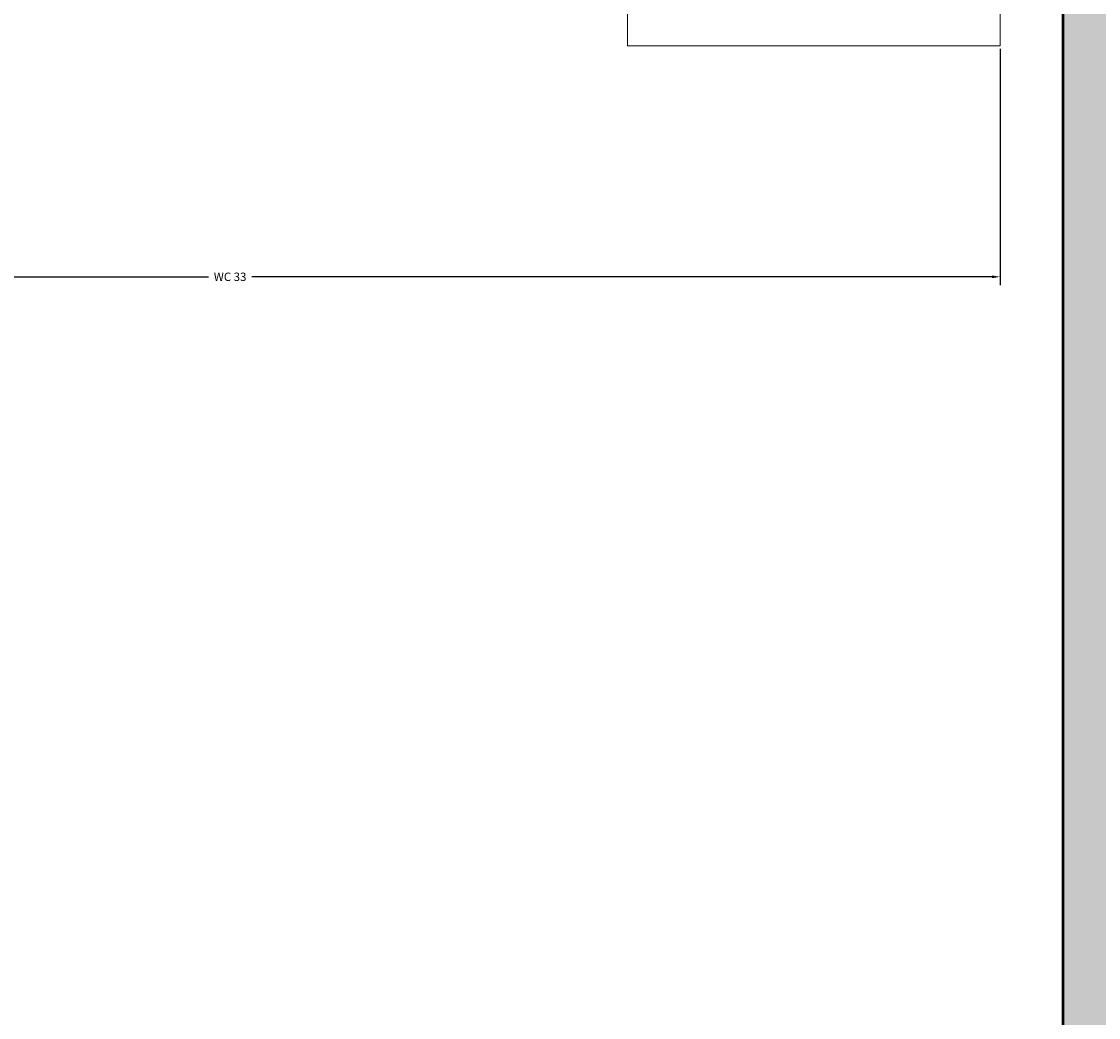
# Model space of a CAD drawing. Units: inches. Extents: x 2231 to 2461, y 2045 to 2455.
# Tile 91 of 95: x 2410 to 2434, y 2383 to 2405. Entities that reach past the tile are written whole.
import ezdxf

# ---------------------------------------------------------------- set-up
doc = ezdxf.new("R2010")
doc.units = ezdxf.units.IN
for name, color, linetype, lineweight in [('A-ANNO-DIMS', 2, 'Continuous', 18), ('A-FLOR-FIXT', 9, 'Continuous', 18), ('A-WALL', 7, 'Continuous', 50)]:
    doc.layers.add(name, color=color, linetype=linetype, lineweight=lineweight)
doc.layers.add('A-WALL-PATT', color=18, linetype='Continuous', lineweight=13, true_color=0x000000)
doc.styles.get("Standard").update_dxf_attribs({"font": 'arial.ttf'})
doc.dimstyles.get("Standard").update_dxf_attribs({"dimtxt": 0.18, "dimasz": 0.18, "dimexe": 0.18, "dimexo": 0.0625, "dimgap": 0.09, "dimtad": 0, "dimtih": 1, "dimtoh": 1, "dimdec": 4, "dimzin": 0, "dimdsep": 46, "dimtxsty": 'Standard', "dimcen": 0.09, "dimadec": 0, "dimazin": 0, "dimtfac": 1, "dimtdec": 4, "dimtofl": 0, "dimtmove": 0, "dimatfit": 3, "dimfxl": 1, "dimtolj": 1, "dimtzin": 0, "dimarcsym": 0})

# ---------------------------------------------------------------- blocks, each defined once
blk = doc.blocks.new('Toilet - top')
blk.add_lwpolyline([(10.5, -8), (10.5, 0), (-10.5, 0), (-10.5, -8)], close=True)
blk = doc.blocks.new('*D21')
at = {"layer": 'A-ANNO-DIMS', "color": 0, "lineweight": -2, "transparency": 16777216}
for p, q in [((2398.404, 2404.126), (2398.404, 2399.052)), ((2431.45, 2404.126), (2431.45, 2399.052)), ((2398.584, 2399.232), (2414.46, 2399.232)), ((2431.27, 2399.232), (2415.394, 2399.232))]:
    blk.add_line(p, q, dxfattribs=at)
at = {"layer": 'A-ANNO-DIMS', "color": 0, "transparency": 16777216}
for points in [[(2398.584, 2399.262), (2398.584, 2399.202), (2398.404, 2399.232)], [(2431.27, 2399.262), (2431.27, 2399.202), (2431.45, 2399.232)]]:
    blk.add_solid(points, dxfattribs=at)
at = {"layer": 'Defpoints', "color": 0, "transparency": 16777216}
for p in [(2398.404, 2404.189), (2431.45, 2404.189), (2431.45, 2399.232)]:
    blk.add_point(p, dxfattribs=at)
at = {"layer": 'A-ANNO-DIMS', "color": 0, "transparency": 16777216, "insert": (2414.927, 2399.232), "char_height": 0.18, "attachment_point": 5}
blk.add_mtext('\\A1;WC 33', dxfattribs=at)
blk = doc.blocks.new('*D38')
at = {"layer": 'A-ANNO-DIMS', "color": 0, "lineweight": -2, "transparency": 16777216}
for p, q in [((2432.856, 2426.833), (2460.606, 2426.833)), ((2460.426, 2426.653), (2460.426, 2381.015)), ((2460.426, 2335.013), (2460.426, 2380.651)), ((2432.856, 2334.833), (2460.606, 2334.833))]:
    blk.add_line(p, q, dxfattribs=at)
at = {"layer": 'A-ANNO-DIMS', "color": 0, "transparency": 16777216}
for points in [[(2460.396, 2426.653), (2460.456, 2426.653), (2460.426, 2426.833)], [(2460.396, 2335.013), (2460.456, 2335.013), (2460.426, 2334.833)]]:
    blk.add_solid(points, dxfattribs=at)
at = {"layer": 'Defpoints', "color": 0, "transparency": 16777216}
for p in [(2432.794, 2426.833), (2460.426, 2426.833), (2432.794, 2334.833)]:
    blk.add_point(p, dxfattribs=at)
at = {"layer": 'A-ANNO-DIMS', "color": 0, "transparency": 16777216, "insert": (2460.426, 2380.833), "char_height": 0.18, "attachment_point": 5}
blk.add_mtext('\\A1;92', dxfattribs=at)
blk = doc.blocks.new('*D42')
at = {"layer": 'A-ANNO-DIMS', "color": 0, "lineweight": -2, "transparency": 16777216}
for p, q in [((2396.794, 2286.895), (2396.794, 2454.645)), ((2432.794, 2286.895), (2432.794, 2454.645)), ((2396.974, 2454.465), (2414.575, 2454.465)), ((2432.614, 2454.465), (2415.012, 2454.465))]:
    blk.add_line(p, q, dxfattribs=at)
at = {"layer": 'A-ANNO-DIMS', "color": 0, "transparency": 16777216}
for points in [[(2396.974, 2454.495), (2396.974, 2454.435), (2396.794, 2454.465)], [(2432.614, 2454.495), (2432.614, 2454.435), (2432.794, 2454.465)]]:
    blk.add_solid(points, dxfattribs=at)
at = {"layer": 'Defpoints', "color": 0, "transparency": 16777216}
for p in [(2432.794, 2454.465), (2396.794, 2286.833), (2432.794, 2286.833)]:
    blk.add_point(p, dxfattribs=at)
at = {"layer": 'A-ANNO-DIMS', "color": 0, "transparency": 16777216, "insert": (2414.794, 2454.465), "char_height": 0.18, "attachment_point": 5}
blk.add_mtext('\\A1;36', dxfattribs=at)
blk = doc.blocks.new('*D59')
at = {"layer": 'A-ANNO-DIMS', "color": 0, "lineweight": -2, "transparency": 16777216}
for p, q in [((2408.794, 2182.895), (2408.794, 2454.645)), ((2432.794, 2182.895), (2432.794, 2454.645)), ((2408.974, 2454.465), (2420.573, 2454.465)), ((2432.614, 2454.465), (2421.014, 2454.465))]:
    blk.add_line(p, q, dxfattribs=at)
at = {"layer": 'A-ANNO-DIMS', "color": 0, "transparency": 16777216}
for points in [[(2408.974, 2454.495), (2408.974, 2454.435), (2408.794, 2454.465)], [(2432.614, 2454.495), (2432.614, 2454.435), (2432.794, 2454.465)]]:
    blk.add_solid(points, dxfattribs=at)
at = {"layer": 'Defpoints', "color": 0, "transparency": 16777216}
for p in [(2432.794, 2454.465), (2408.794, 2182.833), (2432.794, 2182.833)]:
    blk.add_point(p, dxfattribs=at)
at = {"layer": 'A-ANNO-DIMS', "color": 0, "transparency": 16777216, "insert": (2420.794, 2454.465), "char_height": 0.18, "attachment_point": 5}
blk.add_mtext('\\A1;24', dxfattribs=at)

msp = doc.modelspace()

# ---------------------------------------------------------------- hatches: boundary and pattern name
at = {"layer": 'A-WALL-PATT'}
h = msp.add_hatch(color=256, dxfattribs=at)
h.dxf.hatch_style = 1
h.paths.add_polyline_path([(2441.7935, 2269.1535), (2432.7935, 2269.1535), (2432.7935, 2186.8328), (2396.7935, 2186.8328), (2396.7935, 2286.8328), (2394.7935, 2286.8328), (2394.7935, 2186.8328), (2334.7935, 2186.8328), (2334.7935, 2182.8328), (2432.7935, 2182.8328), (2432.7935, 2072.8328), (2416.6639, 2072.8328), (2416.6639, 2063.8328), (2441.7935, 2063.8328)])
h.paths.add_polyline_path([(2368.6639, 2072.8328), (2367.04, 2072.8328), (2330.7942, 2072.8328), (2330.7397, 2063.8328), (2368.6639, 2063.8328)])
h.paths.add_polyline_path([(2300.7392, 2068.3328), (2300.7392, 2072.8328), (2298.7935, 2072.8328), (2294.7935, 2072.8328), (2258.7935, 2072.8328), (2258.7935, 2120.8328), (2294.7935, 2120.8328), (2298.7935, 2120.8328), (2298.7935, 2128.8328), (2294.7935, 2128.8328), (2294.7935, 2124.8328), (2258.7935, 2124.8328), (2258.7935, 2182.8328), (2294.7935, 2182.8328), (2294.7935, 2174.8328), (2298.7935, 2174.8328), (2298.7935, 2182.8328), (2304.7935, 2182.8328), (2304.7935, 2186.8328), (2258.7935, 2186.8328), (2258.7935, 2221.999), (2249.7935, 2221.999), (2249.7935, 2063.8328), (2300.7392, 2063.8328)])
h.paths.add_polyline_path([(2391.9338, 2435.8328), (2333.82, 2435.8328), (2333.82, 2426.8328), (2368.7935, 2426.8328), (2368.7935, 2374.9508), (2368.7935, 2370.8328), (2372.3935, 2370.8328), (2372.7935, 2370.8328), (2372.7935, 2426.8328), (2391.9338, 2426.8328)])
h.paths.add_polyline_path([(2441.7935, 2435.8328), (2415.9338, 2435.8328), (2415.9338, 2426.8328), (2432.7935, 2426.8328), (2432.7935, 2334.8328), (2372.7935, 2334.8328), (2372.7935, 2346.8328), (2368.7935, 2346.8328), (2368.7935, 2306.8328), (2360.7935, 2306.8328), (2360.7935, 2302.8328), (2368.7935, 2302.8328), (2372.7935, 2302.8328), (2372.7935, 2330.8328), (2432.7935, 2330.8328), (2432.7935, 2317.1535), (2441.7935, 2317.1535)])
h.paths.add_polyline_path([(2285.82, 2435.8328), (2249.7935, 2435.8328), (2249.7935, 2269.999), (2258.7935, 2269.999), (2258.7935, 2302.8328), (2318.8168, 2302.8328), (2330.7935, 2302.8328), (2330.7935, 2306.8328), (2258.7935, 2306.8328), (2258.7935, 2426.8328), (2285.82, 2426.8328)])

# ---------------------------------------------------------------- linework, layer by layer
at = {"layer": 'A-WALL'}
msp.add_line((2432.7935, 2426.8328), (2432.7935, 2334.8328), dxfattribs=at)

# ---------------------------------------------------------------- block references
at = {"layer": 'A-FLOR-FIXT', "rotation": 270}
msp.add_blockref('Toilet - top', (2431.4505, 2414.6888), dxfattribs=at)

# ---------------------------------------------------------------- dimensions: what is measured, and where the dimension line sits
at = {"layer": 'A-ANNO-DIMS'}
for p1, p2, picture, middle in [((2396.7935, 2286.8328), (2432.7935, 2286.8328), '*D42', (2414.7935, 2454.4653)), ((2408.7935, 2182.8328), (2432.7935, 2182.8328), '*D59', (2420.7935, 2454.4653))]:
    dim = msp.add_linear_dim(base=(2432.7935, 2454.4653), p1=p1, p2=p2, dimstyle='Standard', override={"dimdec": 0, "dimlfac": 1, "dimrnd": 0, "dimzin": 0, "dimdsep": 46, "dimlunit": 2}, dxfattribs=at)
    dim.commit()
    dim.dimension.update_dxf_attribs({"geometry": picture, "text_midpoint": middle})
dim = msp.add_linear_dim(base=(2460.426, 2426.8328), p1=(2432.7935, 2334.8328), p2=(2432.7935, 2426.8328), angle=90, dimstyle='Standard', override={"dimdec": 0, "dimlfac": 1, "dimrnd": 0, "dimzin": 0, "dimdsep": 46, "dimlunit": 2}, dxfattribs=at)
dim.commit()
dim.dimension.update_dxf_attribs({"geometry": '*D38', "text_midpoint": (2460.426, 2380.8328)})
dim = msp.add_linear_dim(base=(2431.4505, 2399.2319), p1=(2398.4042, 2404.1888), p2=(2431.4505, 2404.1888), text='WC <>', dimstyle='Standard', override={"dimdec": 0, "dimlfac": 1, "dimrnd": 0, "dimzin": 0, "dimdsep": 46, "dimlunit": 2}, dxfattribs=at)
dim.commit()
dim.dimension.update_dxf_attribs({"geometry": '*D21', "text_midpoint": (2414.9274, 2399.2319)})

doc.saveas('drawing.dxf')
